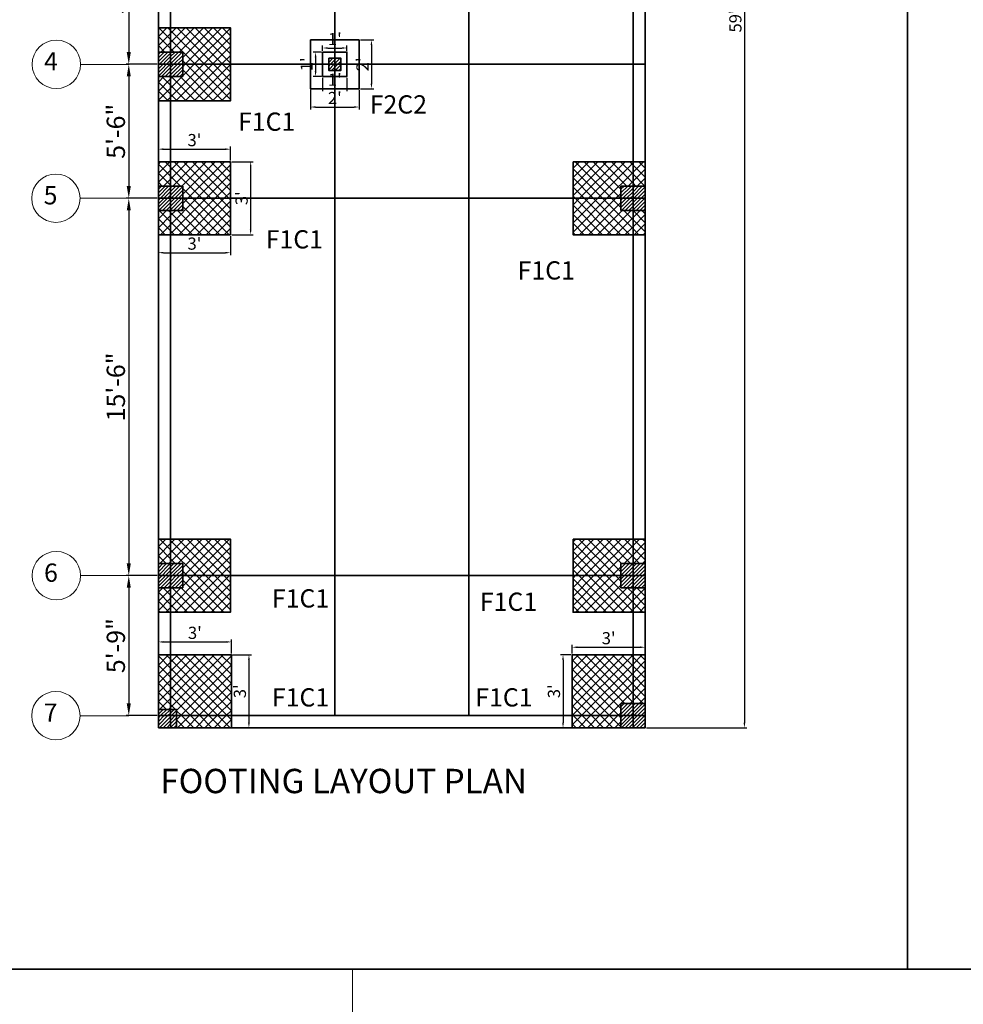
# Model space of a CAD drawing. Units: millimetres. Extents: x 20768 to 23556, y 50760 to 52704.
# Tile 33 of 36: x 22556 to 23021, y 51606 to 52092. Entities that reach past the tile are written whole.
import ezdxf

# ---------------------------------------------------------------- set-up
doc = ezdxf.new("R2010")
doc.units = ezdxf.units.MM
for name, color, linetype, lineweight in [('A-ANNO-SCHD', 7, 'Continuous', 18), ('A-ANNO-TTLB', 7, 'Continuous', 35), ('S-ANNO-DIMS', 2, 'Continuous', 18), ('S-ANNO-TEXT', 6, 'Continuous', 18), ('S-BEAM', 3, 'Continuous', 35), ('S-COLS', 20, 'Continuous', 35), ('S-COLS-PATT', 8, 'Continuous', 13), ('S-FNDN', 200, 'Continuous', 35), ('S-GRID', 1, 'Continuous', 18)]:
    doc.layers.add(name, color=color, linetype=linetype, lineweight=lineweight)
doc.styles.get("Standard").update_dxf_attribs({"font": 'arial.ttf'})
doc.dimstyles.new('ISO-25', dxfattribs={"dimtxt": 6, "dimasz": 2.5, "dimexe": 1.25, "dimexo": 0.625, "dimtad": 1, "dimdec": 0, "dimlunit": 3, "dimtxsty": 'Standard', "dimcen": 2.5, "dimadec": 0, "dimazin": 0, "dimtfac": 1, "dimtdec": 0, "dimtmove": 0, "dimatfit": 3, "dimfxl": 1, "dimarcsym": 0})
pattern_1 = [(45, (568.6884, 0), (-0.898025612, 0.898025612), [])]
pattern_2 = [(45, (-102.8262, 0), (-2.24506403, 2.24506403), []), (135, (-102.8262, 0), (-2.24506403, -2.24506403), [])]
pattern_3 = [(45, (-102.8262, 0), (-0.898025612, 0.898025612), [])]

# ---------------------------------------------------------------- blocks, each defined once
blk = doc.blocks.new('*D56')
at = {"layer": 'Defpoints', "color": 0, "transparency": 16777216}
for p in [(22623.96, 52129.51), (22609.39, 52069.51), (22623.96, 52069.51)]:
    blk.add_point(p, dxfattribs=at)
at = {"layer": 'S-ANNO-DIMS', "color": 0, "lineweight": -2, "transparency": 16777216}
for p, q in [((22623.34, 52129.51), (22608.14, 52129.51)), ((22609.39, 52123.51), (22609.39, 52075.51)), ((22623.34, 52069.51), (22608.14, 52069.51))]:
    blk.add_line(p, q, dxfattribs=at)
at = {"layer": 'S-ANNO-DIMS', "color": 0, "transparency": 16777216}
for points in [[(22608.39, 52123.51), (22610.39, 52123.51), (22609.39, 52129.51)], [(22608.39, 52075.51), (22610.39, 52075.51), (22609.39, 52069.51)]]:
    blk.add_solid(points, dxfattribs=at)
at = {"layer": 'S-ANNO-DIMS', "color": 0, "transparency": 16777216, "insert": (22604.19, 52099.51), "char_height": 9, "attachment_point": 5, "rotation": 90}
blk.add_mtext("5'", dxfattribs=at)
blk = doc.blocks.new('*D57')
at = {"layer": 'Defpoints', "color": 0, "transparency": 16777216}
for p in [(22623.96, 52069.51), (22609.39, 52003.51), (22623.96, 52003.51)]:
    blk.add_point(p, dxfattribs=at)
at = {"layer": 'S-ANNO-DIMS', "color": 0, "lineweight": -2, "transparency": 16777216}
for p, q in [((22623.34, 52069.51), (22608.14, 52069.51)), ((22609.39, 52063.51), (22609.39, 52009.51)), ((22623.34, 52003.51), (22608.14, 52003.51))]:
    blk.add_line(p, q, dxfattribs=at)
at = {"layer": 'S-ANNO-DIMS', "color": 0, "transparency": 16777216}
for points in [[(22608.39, 52063.51), (22610.39, 52063.51), (22609.39, 52069.51)], [(22608.39, 52009.51), (22610.39, 52009.51), (22609.39, 52003.51)]]:
    blk.add_solid(points, dxfattribs=at)
at = {"layer": 'S-ANNO-DIMS', "color": 0, "transparency": 16777216, "insert": (22604.17, 52036.51), "char_height": 9, "attachment_point": 5, "rotation": 90}
blk.add_mtext('5\'-6"', dxfattribs=at)
blk = doc.blocks.new('*D58')
at = {"layer": 'Defpoints', "color": 0, "transparency": 16777216}
for p in [(22623.96, 52003.51), (22609.39, 51817.51), (22623.96, 51817.51)]:
    blk.add_point(p, dxfattribs=at)
at = {"layer": 'S-ANNO-DIMS', "color": 0, "lineweight": -2, "transparency": 16777216}
for p, q in [((22623.34, 52003.51), (22608.14, 52003.51)), ((22609.39, 51997.51), (22609.39, 51823.51)), ((22623.34, 51817.51), (22608.14, 51817.51))]:
    blk.add_line(p, q, dxfattribs=at)
at = {"layer": 'S-ANNO-DIMS', "color": 0, "transparency": 16777216}
for points in [[(22608.39, 51997.51), (22610.39, 51997.51), (22609.39, 52003.51)], [(22608.39, 51823.51), (22610.39, 51823.51), (22609.39, 51817.51)]]:
    blk.add_solid(points, dxfattribs=at)
at = {"layer": 'S-ANNO-DIMS', "color": 0, "transparency": 16777216, "insert": (22604.17, 51910.51), "char_height": 9, "attachment_point": 5, "rotation": 90}
blk.add_mtext('15\'-6"', dxfattribs=at)
blk = doc.blocks.new('*D47')
at = {"layer": 'Defpoints', "color": 0, "transparency": 16777216}
for p in [(22623.96, 51817.51), (22609.39, 51748.51), (22623.96, 51748.51)]:
    blk.add_point(p, dxfattribs=at)
at = {"layer": 'S-ANNO-DIMS', "color": 0, "lineweight": -2, "transparency": 16777216}
for p, q in [((22623.34, 51817.51), (22608.14, 51817.51)), ((22609.39, 51811.51), (22609.39, 51754.51)), ((22623.34, 51748.51), (22608.14, 51748.51))]:
    blk.add_line(p, q, dxfattribs=at)
at = {"layer": 'S-ANNO-DIMS', "color": 0, "transparency": 16777216}
for points in [[(22608.39, 51811.51), (22610.39, 51811.51), (22609.39, 51817.51)], [(22608.39, 51754.51), (22610.39, 51754.51), (22609.39, 51748.51)]]:
    blk.add_solid(points, dxfattribs=at)
at = {"layer": 'S-ANNO-DIMS', "color": 0, "transparency": 16777216, "insert": (22604.17, 51783.01), "char_height": 9, "attachment_point": 5, "rotation": 90}
blk.add_mtext('5\'-9"', dxfattribs=at)
blk = doc.blocks.new('*D68')
at = {"layer": 'Defpoints', "color": 0, "transparency": 16777216}
for p in [(22704.96, 52075.51), (22716.96, 52077.55), (22716.96, 52075.51)]:
    blk.add_point(p, dxfattribs=at)
at = {"layer": 'S-ANNO-DIMS', "color": 0, "lineweight": -2, "transparency": 16777216}
for p, q in [((22704.96, 52076.13), (22704.96, 52078.8)), ((22716.96, 52076.13), (22716.96, 52078.8)), ((22707.46, 52077.55), (22714.46, 52077.55))]:
    blk.add_line(p, q, dxfattribs=at)
at = {"layer": 'S-ANNO-DIMS', "color": 0, "transparency": 16777216}
for points in [[(22707.46, 52077.96), (22707.46, 52077.13), (22704.96, 52077.55)], [(22714.46, 52077.96), (22714.46, 52077.13), (22716.96, 52077.55)]]:
    blk.add_solid(points, dxfattribs=at)
at = {"layer": 'S-ANNO-DIMS', "color": 0, "transparency": 16777216, "insert": (22710.96, 52081.18), "char_height": 6, "attachment_point": 5}
blk.add_mtext("1'", dxfattribs=at)
blk = doc.blocks.new('*D69')
at = {"layer": 'Defpoints', "color": 0, "transparency": 16777216}
for p in [(22722.96, 52081.51), (22722.96, 52057.51), (22729.01, 52057.51)]:
    blk.add_point(p, dxfattribs=at)
at = {"layer": 'S-ANNO-DIMS', "color": 0, "lineweight": -2, "transparency": 16777216}
for p, q in [((22723.59, 52081.51), (22730.26, 52081.51)), ((22729.01, 52079.01), (22729.01, 52060.01)), ((22723.59, 52057.51), (22730.26, 52057.51))]:
    blk.add_line(p, q, dxfattribs=at)
at = {"layer": 'S-ANNO-DIMS', "color": 0, "transparency": 16777216}
for points in [[(22728.59, 52079.01), (22729.42, 52079.01), (22729.01, 52081.51)], [(22728.59, 52060.01), (22729.42, 52060.01), (22729.01, 52057.51)]]:
    blk.add_solid(points, dxfattribs=at)
at = {"layer": 'S-ANNO-DIMS', "color": 0, "transparency": 16777216, "insert": (22725.37, 52069.51), "char_height": 6, "attachment_point": 5, "rotation": 90}
blk.add_mtext("2'", dxfattribs=at)
blk = doc.blocks.new('*D70')
at = {"layer": 'Defpoints', "color": 0, "transparency": 16777216}
for p in [(22698.96, 52057.51), (22722.96, 52057.51), (22722.96, 52048.47)]:
    blk.add_point(p, dxfattribs=at)
at = {"layer": 'S-ANNO-DIMS', "color": 0, "lineweight": -2, "transparency": 16777216}
for p, q in [((22698.96, 52056.88), (22698.96, 52047.22)), ((22722.96, 52056.88), (22722.96, 52047.22)), ((22701.46, 52048.47), (22720.46, 52048.47))]:
    blk.add_line(p, q, dxfattribs=at)
at = {"layer": 'S-ANNO-DIMS', "color": 0, "transparency": 16777216}
for points in [[(22701.46, 52048.89), (22701.46, 52048.06), (22698.96, 52048.47)], [(22720.46, 52048.89), (22720.46, 52048.06), (22722.96, 52048.47)]]:
    blk.add_solid(points, dxfattribs=at)
at = {"layer": 'S-ANNO-DIMS', "color": 0, "transparency": 16777216, "insert": (22710.96, 52052.11), "char_height": 6, "attachment_point": 5}
blk.add_mtext("2'", dxfattribs=at)
blk = doc.blocks.new('*D71')
at = {"layer": 'Defpoints', "color": 0, "transparency": 16777216}
for p in [(22704.96, 52063.51), (22716.96, 52063.51), (22716.96, 52057.51)]:
    blk.add_point(p, dxfattribs=at)
at = {"layer": 'S-ANNO-DIMS', "color": 0, "lineweight": -2, "transparency": 16777216}
for p, q in [((22704.96, 52062.88), (22704.96, 52056.26)), ((22716.96, 52062.88), (22716.96, 52056.26)), ((22707.46, 52057.51), (22714.46, 52057.51))]:
    blk.add_line(p, q, dxfattribs=at)
at = {"layer": 'S-ANNO-DIMS', "color": 0, "transparency": 16777216}
for points in [[(22707.46, 52057.93), (22707.46, 52057.09), (22704.96, 52057.51)], [(22714.46, 52057.93), (22714.46, 52057.09), (22716.96, 52057.51)]]:
    blk.add_solid(points, dxfattribs=at)
at = {"layer": 'S-ANNO-DIMS', "color": 0, "transparency": 16777216, "insert": (22710.96, 52061.15), "char_height": 6, "attachment_point": 5}
blk.add_mtext("1'", dxfattribs=at)
blk = doc.blocks.new('*D50')
at = {"layer": 'Defpoints', "color": 0, "transparency": 16777216}
for p in [(22704.96, 52075.51), (22701.48, 52063.51), (22704.96, 52063.51)]:
    blk.add_point(p, dxfattribs=at)
at = {"layer": 'S-ANNO-DIMS', "color": 0, "lineweight": -2, "transparency": 16777216}
for p, q in [((22704.34, 52075.51), (22700.23, 52075.51)), ((22701.48, 52073.01), (22701.48, 52066.01)), ((22704.34, 52063.51), (22700.23, 52063.51))]:
    blk.add_line(p, q, dxfattribs=at)
at = {"layer": 'S-ANNO-DIMS', "color": 0, "transparency": 16777216}
for points in [[(22701.07, 52073.01), (22701.9, 52073.01), (22701.48, 52075.51)], [(22701.07, 52066.01), (22701.9, 52066.01), (22701.48, 52063.51)]]:
    blk.add_solid(points, dxfattribs=at)
at = {"layer": 'S-ANNO-DIMS', "color": 0, "transparency": 16777216, "insert": (22697.85, 52069.51), "char_height": 6, "attachment_point": 5, "rotation": 90}
blk.add_mtext("1'", dxfattribs=at)
blk = doc.blocks.new('*D72')
at = {"layer": 'Defpoints', "color": 0, "transparency": 16777216}
for p in [(22659.96, 51784.85), (22623.96, 51778.51), (22659.96, 51778.51)]:
    blk.add_point(p, dxfattribs=at)
at = {"layer": 'S-ANNO-DIMS', "color": 0, "lineweight": -2, "transparency": 16777216}
for p, q in [((22623.96, 51779.13), (22623.96, 51786.1)), ((22626.46, 51784.85), (22657.46, 51784.85)), ((22659.96, 51779.13), (22659.96, 51786.1))]:
    blk.add_line(p, q, dxfattribs=at)
at = {"layer": 'S-ANNO-DIMS', "color": 0, "transparency": 16777216}
for points in [[(22626.46, 51785.26), (22626.46, 51784.43), (22623.96, 51784.85)], [(22657.46, 51785.26), (22657.46, 51784.43), (22659.96, 51784.85)]]:
    blk.add_solid(points, dxfattribs=at)
at = {"layer": 'S-ANNO-DIMS', "color": 0, "transparency": 16777216, "insert": (22641.96, 51788.54), "char_height": 6, "attachment_point": 5}
blk.add_mtext("3'", dxfattribs=at)
blk = doc.blocks.new('*D73')
at = {"layer": 'Defpoints', "color": 0, "transparency": 16777216}
for p in [(22659.96, 51778.51), (22659.96, 51742.51), (22668.62, 51742.51)]:
    blk.add_point(p, dxfattribs=at)
at = {"layer": 'S-ANNO-DIMS', "color": 0, "lineweight": -2, "transparency": 16777216}
for p, q in [((22660.59, 51778.51), (22669.87, 51778.51)), ((22668.62, 51776.01), (22668.62, 51745.01)), ((22660.59, 51742.51), (22669.87, 51742.51))]:
    blk.add_line(p, q, dxfattribs=at)
at = {"layer": 'S-ANNO-DIMS', "color": 0, "transparency": 16777216}
for points in [[(22668.2, 51776.01), (22669.04, 51776.01), (22668.62, 51778.51)], [(22668.2, 51745.01), (22669.04, 51745.01), (22668.62, 51742.51)]]:
    blk.add_solid(points, dxfattribs=at)
at = {"layer": 'S-ANNO-DIMS', "color": 0, "transparency": 16777216, "insert": (22664.93, 51760.51), "char_height": 6, "attachment_point": 5, "rotation": 90}
blk.add_mtext("3'", dxfattribs=at)
blk = doc.blocks.new('*D74')
at = {"layer": 'Defpoints', "color": 0, "transparency": 16777216}
for p in [(22863.96, 51782.23), (22827.96, 51778.51), (22863.96, 51778.51)]:
    blk.add_point(p, dxfattribs=at)
at = {"layer": 'S-ANNO-DIMS', "color": 0, "lineweight": -2, "transparency": 16777216}
for p, q in [((22827.96, 51779.13), (22827.96, 51783.48)), ((22830.46, 51782.23), (22861.46, 51782.23)), ((22863.96, 51779.13), (22863.96, 51783.48))]:
    blk.add_line(p, q, dxfattribs=at)
at = {"layer": 'S-ANNO-DIMS', "color": 0, "transparency": 16777216}
for points in [[(22830.46, 51782.64), (22830.46, 51781.81), (22827.96, 51782.23)], [(22861.46, 51782.64), (22861.46, 51781.81), (22863.96, 51782.23)]]:
    blk.add_solid(points, dxfattribs=at)
at = {"layer": 'S-ANNO-DIMS', "color": 0, "transparency": 16777216, "insert": (22845.96, 51785.92), "char_height": 6, "attachment_point": 5}
blk.add_mtext("3'", dxfattribs=at)
blk = doc.blocks.new('*D75')
at = {"layer": 'Defpoints', "color": 0, "transparency": 16777216}
for p in [(22827.96, 51778.51), (22823.46, 51742.51), (22827.96, 51742.51)]:
    blk.add_point(p, dxfattribs=at)
at = {"layer": 'S-ANNO-DIMS', "color": 0, "lineweight": -2, "transparency": 16777216}
for p, q in [((22827.34, 51778.51), (22822.21, 51778.51)), ((22823.46, 51776.01), (22823.46, 51745.01)), ((22827.34, 51742.51), (22822.21, 51742.51))]:
    blk.add_line(p, q, dxfattribs=at)
at = {"layer": 'S-ANNO-DIMS', "color": 0, "transparency": 16777216}
for points in [[(22823.04, 51776.01), (22823.88, 51776.01), (22823.46, 51778.51)], [(22823.04, 51745.01), (22823.88, 51745.01), (22823.46, 51742.51)]]:
    blk.add_solid(points, dxfattribs=at)
at = {"layer": 'S-ANNO-DIMS', "color": 0, "transparency": 16777216, "insert": (22819.77, 51760.51), "char_height": 6, "attachment_point": 5, "rotation": 90}
blk.add_mtext("3'", dxfattribs=at)
blk = doc.blocks.new('*D76')
at = {"layer": 'Defpoints', "color": 0, "transparency": 16777216}
for p in [(22659.53, 52027.69), (22623.96, 52021.51), (22659.53, 52021.51)]:
    blk.add_point(p, dxfattribs=at)
at = {"layer": 'S-ANNO-DIMS', "color": 0, "lineweight": -2, "transparency": 16777216}
for p, q in [((22623.96, 52022.13), (22623.96, 52028.94)), ((22626.46, 52027.69), (22657.03, 52027.69)), ((22659.53, 52022.13), (22659.53, 52028.94))]:
    blk.add_line(p, q, dxfattribs=at)
at = {"layer": 'S-ANNO-DIMS', "color": 0, "transparency": 16777216}
for points in [[(22626.46, 52028.11), (22626.46, 52027.28), (22623.96, 52027.69)], [(22657.03, 52028.11), (22657.03, 52027.28), (22659.53, 52027.69)]]:
    blk.add_solid(points, dxfattribs=at)
at = {"layer": 'S-ANNO-DIMS', "color": 0, "transparency": 16777216, "insert": (22641.75, 52031.39), "char_height": 6, "attachment_point": 5}
blk.add_mtext("3'", dxfattribs=at)
blk = doc.blocks.new('*D77')
at = {"layer": 'Defpoints', "color": 0, "transparency": 16777216}
for p in [(22659.53, 52021.51), (22659.53, 51985.51), (22669.47, 51985.51)]:
    blk.add_point(p, dxfattribs=at)
at = {"layer": 'S-ANNO-DIMS', "color": 0, "lineweight": -2, "transparency": 16777216}
for p, q in [((22660.16, 52021.51), (22670.72, 52021.51)), ((22669.47, 52019.01), (22669.47, 51988.01)), ((22660.16, 51985.51), (22670.72, 51985.51))]:
    blk.add_line(p, q, dxfattribs=at)
at = {"layer": 'S-ANNO-DIMS', "color": 0, "transparency": 16777216}
for points in [[(22669.05, 52019.01), (22669.89, 52019.01), (22669.47, 52021.51)], [(22669.05, 51988.01), (22669.89, 51988.01), (22669.47, 51985.51)]]:
    blk.add_solid(points, dxfattribs=at)
at = {"layer": 'S-ANNO-DIMS', "color": 0, "transparency": 16777216, "insert": (22665.78, 52003.51), "char_height": 6, "attachment_point": 5, "rotation": 90}
blk.add_mtext("3'", dxfattribs=at)
blk = doc.blocks.new('*D78')
at = {"layer": 'Defpoints', "color": 0, "transparency": 16777216}
for p in [(22623.96, 51985.51), (22659.53, 51985.51), (22659.53, 51976.68)]:
    blk.add_point(p, dxfattribs=at)
at = {"layer": 'S-ANNO-DIMS', "color": 0, "lineweight": -2, "transparency": 16777216}
for p, q in [((22623.96, 51984.88), (22623.96, 51975.43)), ((22659.53, 51984.88), (22659.53, 51975.43)), ((22626.46, 51976.68), (22657.03, 51976.68))]:
    blk.add_line(p, q, dxfattribs=at)
at = {"layer": 'S-ANNO-DIMS', "color": 0, "transparency": 16777216}
for points in [[(22626.46, 51977.1), (22626.46, 51976.27), (22623.96, 51976.68)], [(22657.03, 51977.1), (22657.03, 51976.27), (22659.53, 51976.68)]]:
    blk.add_solid(points, dxfattribs=at)
at = {"layer": 'S-ANNO-DIMS', "color": 0, "transparency": 16777216, "insert": (22641.75, 51980.37), "char_height": 6, "attachment_point": 5}
blk.add_mtext("3'", dxfattribs=at)
blk = doc.blocks.new('GRID-BUBBLE')
blk.add_line((47.87, 11.93), (23.87, 11.93))
blk.add_circle((11.93, 11.93), 11.93)
blk = doc.blocks.new('*D226')
at = {"layer": 'Defpoints', "color": 0, "transparency": 16777216}
for p in [(22863.96, 52450.51), (22863.96, 51742.51), (22912.89, 51742.51)]:
    blk.add_point(p, dxfattribs=at)
at = {"layer": 'S-ANNO-DIMS', "color": 0, "lineweight": -2, "transparency": 16777216}
for p, q in [((22864.59, 52450.51), (22914.14, 52450.51)), ((22912.89, 52448.01), (22912.89, 51745.01)), ((22864.59, 51742.51), (22914.14, 51742.51))]:
    blk.add_line(p, q, dxfattribs=at)
at = {"layer": 'S-ANNO-DIMS', "color": 0, "transparency": 16777216}
for points in [[(22912.48, 52448.01), (22913.31, 52448.01), (22912.89, 52450.51)], [(22912.48, 51745.01), (22913.31, 51745.01), (22912.89, 51742.51)]]:
    blk.add_solid(points, dxfattribs=at)
at = {"layer": 'S-ANNO-DIMS', "color": 0, "transparency": 16777216, "insert": (22909.21, 52096.51), "char_height": 6, "attachment_point": 5, "rotation": 90}
blk.add_mtext('59\'-0"', dxfattribs=at)

msp = doc.modelspace()

# ---------------------------------------------------------------- hatches: boundary and pattern name
at = {"layer": 'S-COLS-PATT'}
h = msp.add_hatch(dxfattribs=at)
h.set_pattern_fill('ANSI37', color=256)
h.set_pattern_definition(pattern_2)
h.paths.add_polyline_path([(22629.96, 52087.51), (22623.96, 52087.51), (22623.96, 52075.51), (22629.96, 52075.51)])
h = msp.add_hatch(dxfattribs=at)
h.set_pattern_fill('ANSI37', color=256)
h.set_pattern_definition(pattern_2)
h.paths.add_polyline_path([(22659.53, 52087.51), (22629.96, 52087.51), (22629.96, 52075.51), (22635.96, 52075.51), (22635.96, 52069.51), (22659.53, 52069.51)])
h = msp.add_hatch(dxfattribs=at)
h.set_pattern_fill('ANSI31', color=256, scale=0.4)
h.set_pattern_definition(pattern_1)
h.paths.add_polyline_path([(22629.96, 52075.51), (22623.96, 52075.51), (22623.96, 52063.51), (22629.96, 52063.51)])
h = msp.add_hatch(dxfattribs=at)
h.set_pattern_fill('ANSI31', color=256, scale=0.4)
h.set_pattern_definition(pattern_1)
h.paths.add_polyline_path([(22635.96, 52075.51), (22629.96, 52075.51), (22629.96, 52069.51), (22635.96, 52069.51)])
h = msp.add_hatch(dxfattribs=at)
h.set_pattern_fill('ANSI31', color=256, scale=0.4)
h.set_pattern_definition(pattern_1)
h.paths.add_polyline_path([(22635.96, 52069.51), (22629.96, 52069.51), (22629.96, 52063.51), (22635.96, 52063.51)])
h = msp.add_hatch(dxfattribs=at)
h.set_pattern_fill('ANSI37', color=256)
h.set_pattern_definition(pattern_2)
h.paths.add_polyline_path([(22659.53, 52069.51), (22635.96, 52069.51), (22635.96, 52063.51), (22629.96, 52063.51), (22629.96, 52051.51), (22659.53, 52051.51)])
h = msp.add_hatch(dxfattribs=at)
h.set_pattern_fill('ANSI31', color=256, scale=0.4)
h.set_pattern_definition(pattern_1)
h.paths.add_polyline_path([(22710.96, 52072.51), (22707.96, 52072.51), (22707.96, 52069.51), (22710.96, 52069.51)])
h = msp.add_hatch(dxfattribs=at)
h.set_pattern_fill('ANSI31', color=256, scale=0.4)
h.set_pattern_definition(pattern_1)
h.paths.add_polyline_path([(22710.96, 52069.51), (22707.96, 52069.51), (22707.96, 52066.51), (22710.96, 52066.51)])
h = msp.add_hatch(dxfattribs=at)
h.set_pattern_fill('ANSI31', color=256, scale=0.4)
h.set_pattern_definition(pattern_1)
h.paths.add_polyline_path([(22713.96, 52072.51), (22710.96, 52072.51), (22710.96, 52069.51), (22713.96, 52069.51)], flags=17)
h = msp.add_hatch(dxfattribs=at)
h.set_pattern_fill('ANSI31', color=256, scale=0.4)
h.set_pattern_definition(pattern_1)
h.paths.add_polyline_path([(22713.96, 52069.51), (22710.96, 52069.51), (22710.96, 52066.51), (22713.96, 52066.51)])
h = msp.add_hatch(dxfattribs=at)
h.set_pattern_fill('ANSI37', color=256)
h.set_pattern_definition(pattern_2)
h.paths.add_polyline_path([(22629.96, 52063.51), (22623.96, 52063.51), (22623.96, 52051.51), (22629.96, 52051.51)])
h = msp.add_hatch(dxfattribs=at)
h.set_pattern_fill('ANSI37', color=256)
h.set_pattern_definition(pattern_2)
h.paths.add_polyline_path([(22629.96, 52021.51), (22623.96, 52021.51), (22623.96, 52009.51), (22629.96, 52009.51)])
h = msp.add_hatch(dxfattribs=at)
h.set_pattern_fill('ANSI37', color=256)
h.set_pattern_definition(pattern_2)
h.paths.add_polyline_path([(22659.53, 52021.51), (22629.96, 52021.51), (22629.96, 52009.51), (22635.96, 52009.51), (22635.96, 52003.51), (22659.53, 52003.51)])
h = msp.add_hatch(dxfattribs=at)
h.set_pattern_fill('ANSI37', color=256)
h.set_pattern_definition(pattern_2)
h.paths.add_polyline_path([(22857.96, 52021.51), (22828.39, 52021.51), (22828.39, 52003.51), (22851.96, 52003.51), (22851.96, 52009.51), (22857.96, 52009.51)])
h = msp.add_hatch(dxfattribs=at)
h.set_pattern_fill('ANSI37', color=256)
h.set_pattern_definition(pattern_2)
h.paths.add_polyline_path([(22863.96, 52021.51), (22857.96, 52021.51), (22857.96, 52009.51), (22863.96, 52009.51)])
h = msp.add_hatch(dxfattribs=at)
h.set_pattern_fill('ANSI31', color=256, scale=0.4)
h.set_pattern_definition(pattern_1)
h.paths.add_polyline_path([(22629.96, 52009.51), (22623.96, 52009.51), (22623.96, 51997.51), (22629.96, 51997.51)])
h = msp.add_hatch(dxfattribs=at)
h.set_pattern_fill('ANSI31', color=256, scale=0.4)
h.set_pattern_definition(pattern_1)
h.paths.add_polyline_path([(22635.96, 52009.51), (22629.96, 52009.51), (22629.96, 52003.51), (22635.96, 52003.51)])
h = msp.add_hatch(dxfattribs=at)
h.set_pattern_fill('ANSI31', color=256, scale=0.4)
h.set_pattern_definition(pattern_1)
h.paths.add_polyline_path([(22857.96, 52009.51), (22851.96, 52009.51), (22851.96, 52003.51), (22857.96, 52003.51)])
h = msp.add_hatch(dxfattribs=at)
h.set_pattern_fill('ANSI31', color=256, scale=0.4)
h.set_pattern_definition(pattern_1)
h.paths.add_polyline_path([(22863.96, 52009.51), (22857.96, 52009.51), (22857.96, 52003.51), (22863.96, 52003.51)])
h = msp.add_hatch(dxfattribs=at)
h.set_pattern_fill('ANSI31', color=256, scale=0.4)
h.set_pattern_definition(pattern_1)
h.paths.add_polyline_path([(22635.96, 52003.51), (22629.96, 52003.51), (22629.96, 51997.51), (22635.96, 51997.51)])
h = msp.add_hatch(dxfattribs=at)
h.set_pattern_fill('ANSI37', color=256)
h.set_pattern_definition(pattern_2)
h.paths.add_polyline_path([(22659.53, 52003.51), (22635.96, 52003.51), (22635.96, 51997.51), (22629.96, 51997.51), (22629.96, 51985.51), (22659.53, 51985.51)])
h = msp.add_hatch(dxfattribs=at)
h.set_pattern_fill('ANSI37', color=256)
h.set_pattern_definition(pattern_2)
h.paths.add_polyline_path([(22857.96, 51997.51), (22851.96, 51997.51), (22851.96, 52003.51), (22828.39, 52003.51), (22828.39, 51985.51), (22857.96, 51985.51)])
h = msp.add_hatch(dxfattribs=at)
h.set_pattern_fill('ANSI31', color=256, scale=0.4)
h.set_pattern_definition(pattern_1)
h.paths.add_polyline_path([(22857.96, 52003.51), (22851.96, 52003.51), (22851.96, 51997.51), (22857.96, 51997.51)])
h = msp.add_hatch(dxfattribs=at)
h.set_pattern_fill('ANSI31', color=256, scale=0.4)
h.set_pattern_definition(pattern_1)
h.paths.add_polyline_path([(22863.96, 52003.51), (22857.96, 52003.51), (22857.96, 51997.51), (22863.96, 51997.51)])
h = msp.add_hatch(dxfattribs=at)
h.set_pattern_fill('ANSI37', color=256)
h.set_pattern_definition(pattern_2)
h.paths.add_polyline_path([(22629.96, 51997.51), (22623.96, 51997.51), (22623.96, 51985.51), (22629.96, 51985.51)])
h = msp.add_hatch(dxfattribs=at)
h.set_pattern_fill('ANSI37', color=256)
h.set_pattern_definition(pattern_2)
h.paths.add_polyline_path([(22863.96, 51997.51), (22857.96, 51997.51), (22857.96, 51985.51), (22863.96, 51985.51)])
h = msp.add_hatch(dxfattribs=at)
h.set_pattern_fill('ANSI37', color=256)
h.set_pattern_definition(pattern_2)
h.paths.add_polyline_path([(22629.96, 51835.51), (22623.96, 51835.51), (22623.96, 51823.51), (22629.96, 51823.51)])
h = msp.add_hatch(dxfattribs=at)
h.set_pattern_fill('ANSI37', color=256)
h.set_pattern_definition(pattern_2)
h.paths.add_polyline_path([(22659.53, 51835.51), (22629.96, 51835.51), (22629.96, 51823.51), (22635.96, 51823.51), (22635.96, 51817.51), (22659.53, 51817.51)])
h = msp.add_hatch(dxfattribs=at)
h.set_pattern_fill('ANSI37', color=256)
h.set_pattern_definition(pattern_2)
h.paths.add_polyline_path([(22857.96, 51835.51), (22828.39, 51835.51), (22828.39, 51817.51), (22851.96, 51817.51), (22851.96, 51823.51), (22857.96, 51823.51)])
h = msp.add_hatch(dxfattribs=at)
h.set_pattern_fill('ANSI37', color=256)
h.set_pattern_definition(pattern_2)
h.paths.add_polyline_path([(22863.96, 51835.51), (22857.96, 51835.51), (22857.96, 51823.51), (22863.96, 51823.51)])
h = msp.add_hatch(dxfattribs=at)
h.set_pattern_fill('ANSI31', color=256, scale=0.4)
h.set_pattern_definition(pattern_1)
h.paths.add_polyline_path([(22629.96, 51823.51), (22623.96, 51823.51), (22623.96, 51811.51), (22629.96, 51811.51)])
h = msp.add_hatch(dxfattribs=at)
h.set_pattern_fill('ANSI31', color=256, scale=0.4)
h.set_pattern_definition(pattern_1)
h.paths.add_polyline_path([(22635.96, 51823.51), (22629.96, 51823.51), (22629.96, 51817.51), (22635.96, 51817.51)])
h = msp.add_hatch(dxfattribs=at)
h.set_pattern_fill('ANSI31', color=256, scale=0.4)
h.set_pattern_definition(pattern_1)
h.paths.add_polyline_path([(22863.96, 51823.51), (22851.96, 51823.51), (22851.96, 51811.51), (22863.96, 51811.51)])
h = msp.add_hatch(dxfattribs=at)
h.set_pattern_fill('ANSI31', color=256, scale=0.4)
h.set_pattern_definition(pattern_1)
h.paths.add_polyline_path([(22635.96, 51817.51), (22629.96, 51817.51), (22629.96, 51811.51), (22635.96, 51811.51)])
h = msp.add_hatch(dxfattribs=at)
h.set_pattern_fill('ANSI37', color=256)
h.set_pattern_definition(pattern_2)
h.paths.add_polyline_path([(22659.53, 51817.51), (22635.96, 51817.51), (22635.96, 51811.51), (22629.96, 51811.51), (22629.96, 51799.51), (22659.53, 51799.51)])
h = msp.add_hatch(dxfattribs=at)
h.set_pattern_fill('ANSI37', color=256)
h.set_pattern_definition(pattern_2)
h.paths.add_polyline_path([(22857.96, 51811.51), (22851.96, 51811.51), (22851.96, 51817.51), (22828.39, 51817.51), (22828.39, 51799.51), (22857.96, 51799.51)])
h = msp.add_hatch(dxfattribs=at)
h.set_pattern_fill('ANSI37', color=256)
h.set_pattern_definition(pattern_2)
h.paths.add_polyline_path([(22629.96, 51811.51), (22623.96, 51811.51), (22623.96, 51799.51), (22629.96, 51799.51)])
h = msp.add_hatch(dxfattribs=at)
h.set_pattern_fill('ANSI37', color=256)
h.set_pattern_definition(pattern_2)
h.paths.add_polyline_path([(22863.96, 51811.51), (22857.96, 51811.51), (22857.96, 51799.51), (22863.96, 51799.51)])
h = msp.add_hatch(dxfattribs=at)
h.set_pattern_fill('ANSI37', color=256)
h.set_pattern_definition(pattern_2)
h.paths.add_polyline_path([(22629.96, 51778.51), (22623.96, 51778.51), (22623.96, 51751.51), (22629.96, 51751.51)])
h = msp.add_hatch(dxfattribs=at)
h.set_pattern_fill('ANSI37', color=256)
h.set_pattern_definition(pattern_2)
h.paths.add_polyline_path([(22659.96, 51778.51), (22629.96, 51778.51), (22629.96, 51751.51), (22632.96, 51751.51), (22632.96, 51748.51), (22659.96, 51748.51)])
h = msp.add_hatch(dxfattribs=at)
h.set_pattern_fill('ANSI37', color=256)
h.set_pattern_definition(pattern_2)
h.paths.add_polyline_path([(22857.96, 51778.51), (22827.96, 51778.51), (22827.96, 51748.51), (22851.96, 51748.51), (22851.96, 51754.51), (22857.96, 51754.51)])
h = msp.add_hatch(dxfattribs=at)
h.set_pattern_fill('ANSI37', color=256)
h.set_pattern_definition(pattern_2)
h.paths.add_polyline_path([(22863.96, 51778.51), (22857.96, 51778.51), (22857.96, 51754.51), (22863.96, 51754.51)])
h = msp.add_hatch(dxfattribs=at)
h.set_pattern_fill('ANSI31', color=256, scale=0.4)
h.set_pattern_definition(pattern_1)
h.paths.add_polyline_path([(22863.96, 51754.51), (22851.96, 51754.51), (22851.96, 51742.51), (22863.96, 51742.51)])
h = msp.add_hatch(dxfattribs=at)
h.set_pattern_fill('ANSI31', color=256, scale=0.4)
h.set_pattern_definition(pattern_3)
h.paths.add_polyline_path([(22629.96, 51751.51), (22623.96, 51751.51), (22623.96, 51748.51), (22629.96, 51748.51)])
h = msp.add_hatch(dxfattribs=at)
h.set_pattern_fill('ANSI31', color=256, scale=0.4)
h.set_pattern_definition(pattern_3)
h.paths.add_polyline_path([(22629.96, 51748.51), (22623.96, 51748.51), (22623.96, 51742.51), (22629.96, 51742.51)])
h = msp.add_hatch(dxfattribs=at)
h.set_pattern_fill('ANSI31', color=256, scale=0.4)
h.set_pattern_definition(pattern_3)
h.paths.add_polyline_path([(22632.96, 51751.51), (22629.96, 51751.51), (22629.96, 51748.51), (22632.96, 51748.51)])
h = msp.add_hatch(dxfattribs=at)
h.set_pattern_fill('ANSI31', color=256, scale=0.4)
h.set_pattern_definition(pattern_3)
h.paths.add_polyline_path([(22632.96, 51748.51), (22629.96, 51748.51), (22629.96, 51742.51), (22632.96, 51742.51)])
h = msp.add_hatch(dxfattribs=at)
h.set_pattern_fill('ANSI37', color=256)
h.set_pattern_definition(pattern_2)
h.paths.add_polyline_path([(22659.96, 51748.51), (22632.96, 51748.51), (22632.96, 51742.51), (22659.96, 51742.51)])
h = msp.add_hatch(dxfattribs=at)
h.set_pattern_fill('ANSI37', color=256)
h.set_pattern_definition(pattern_2)
h.paths.add_polyline_path([(22851.96, 51748.51), (22827.96, 51748.51), (22827.96, 51742.51), (22851.96, 51742.51)])

# ---------------------------------------------------------------- linework, layer by layer
at = {"layer": 'A-ANNO-SCHD'}
msp.add_line((22719.7, 51623.53), (22719.7, 50975.78), dxfattribs=at)
at = {"layer": 'A-ANNO-TTLB'}
msp.add_line((22993.36, 52703.98), (22993.36, 51623.53), dxfattribs=at)
msp.add_lwpolyline([(20768.14, 52703.98), (23555.8, 52703.98), (23555.8, 51623.53), (20768.14, 51623.53)], close=True, dxfattribs=at)
at = {"layer": 'S-BEAM'}
for p, q in [((22710.96, 52450.51), (22710.96, 51748.51)), ((22776.96, 52450.51), (22776.96, 51748.51)), ((22629.96, 52444.51), (22629.96, 51742.51)), ((22857.96, 52135.51), (22857.96, 51823.51)), ((22623.96, 52069.51), (22863.96, 52069.51)), ((22623.96, 52003.51), (22863.96, 52003.51)), ((22857.96, 51823.51), (22857.96, 51742.51)), ((22623.96, 51817.51), (22863.96, 51817.51)), ((22623.96, 51748.51), (22863.96, 51748.51))]:
    msp.add_line(p, q, dxfattribs=at)
at = {"layer": 'S-COLS'}
for points in [[(22623.96, 52087.51), (22659.53, 52087.51), (22659.53, 52051.51), (22623.96, 52051.51)], [(22698.96, 52081.51), (22722.96, 52081.51), (22722.96, 52057.51), (22698.96, 52057.51)], [(22635.96, 52075.51), (22623.96, 52075.51), (22623.96, 52063.51), (22635.96, 52063.51)], [(22704.96, 52075.51), (22716.96, 52075.51), (22716.96, 52063.51), (22704.96, 52063.51)], [(22707.96, 52072.51), (22713.96, 52072.51), (22713.96, 52066.51), (22707.96, 52066.51)], [(22623.96, 52021.51), (22659.53, 52021.51), (22659.53, 51985.51), (22623.96, 51985.51)], [(22828.39, 52021.51), (22863.96, 52021.51), (22863.96, 51985.51), (22828.39, 51985.51)], [(22635.96, 52009.51), (22623.96, 52009.51), (22623.96, 51997.51), (22635.96, 51997.51)], [(22851.96, 52009.51), (22863.96, 52009.51), (22863.96, 51997.51), (22851.96, 51997.51)], [(22623.96, 51835.51), (22659.53, 51835.51), (22659.53, 51799.51), (22623.96, 51799.51)], [(22828.39, 51835.51), (22863.96, 51835.51), (22863.96, 51799.51), (22828.39, 51799.51)], [(22635.96, 51823.51), (22623.96, 51823.51), (22623.96, 51811.51), (22635.96, 51811.51)], [(22851.96, 51823.51), (22863.96, 51823.51), (22863.96, 51811.51), (22851.96, 51811.51)], [(22623.96, 51742.51), (22659.96, 51742.51), (22659.96, 51778.51), (22623.96, 51778.51)], [(22863.96, 51742.51), (22827.96, 51742.51), (22827.96, 51778.51), (22863.96, 51778.51)], [(22851.96, 51754.51), (22863.96, 51754.51), (22863.96, 51742.51), (22851.96, 51742.51)], [(22623.96, 51742.51), (22632.96, 51742.51), (22632.96, 51751.51), (22623.96, 51751.51)]]:
    msp.add_lwpolyline(points, close=True, dxfattribs=at)
at = {"layer": 'S-FNDN'}
for p, q in [((22623.96, 52450.51), (22623.96, 51742.51)), ((22863.96, 52450.51), (22863.96, 51742.51)), ((22623.96, 51742.51), (22863.96, 51742.51))]:
    msp.add_line(p, q, dxfattribs=at)

# ---------------------------------------------------------------- block references
at = {"layer": 'S-GRID'}
for p in [(22561.73, 52057.57), (22561.52, 51991.57), (22561.73, 51805.57), (22561.52, 51736.57)]:
    msp.add_blockref('GRID-BUBBLE', p, dxfattribs=at)

# ---------------------------------------------------------------- texts
at = {"layer": 'S-ANNO-TEXT', "attachment_point": 1}
for s, width, insert, char_height in [('  4', 27.5349, (22562.12, 52075.48), 9), ('F2C2', 26.4582, (22728.17, 52054.25), 9), ('F1C1', 26.4582, (22663.26, 52045.76), 9), ('  5', 27.5349, (22561.91, 52009.48), 9), ('F1C1', 26.4582, (22676.89, 51987.76), 9), ('F1C1', 26.4582, (22801.08, 51972.45), 9), ('  6', 27.5349, (22562.12, 51823.48), 9), ('F1C1', 26.4582, (22679.94, 51810.8), 9), ('F1C1', 26.4582, (22782.47, 51809.16), 9), ('F1C1', 26.4582, (22679.94, 51762.02), 9), ('F1C1', 26.4582, (22780.21, 51762.02), 9), ('  7', 27.5349, (22561.91, 51754.48), 9), ('FOOTING LAYOUT PLAN', 241.5904, (22624.93, 51722.3), 12)]:
    msp.add_mtext_dynamic_manual_height_columns(s, width=width, gutter_width=12.5, heights=[0], dxfattribs=dict(at, insert=insert, char_height=char_height))

# ---------------------------------------------------------------- dimensions: what is measured, and where the dimension line sits
at = {"layer": 'S-ANNO-DIMS'}
for base, p1, p2, override, picture, middle in [((22912.89, 51742.51), (22863.96, 52450.51), (22863.96, 51742.51), {"dimdec": 1, "dimlfac": 1, "dimrnd": 0, "dimzin": 1, "dimdsep": 46, "dimlunit": 4, "dimfrac": 2}, '*D226', (22909.21, 52096.51)), ((22609.39, 52069.51), (22623.96, 52129.51), (22623.96, 52069.51), {"dimtxt": 9, "dimasz": 6, "dimclrd": 0, "dimclre": 0, "dimclrt": 0}, '*D56', (22604.19, 52099.51)), ((22729.01, 52057.51), (22722.96, 52081.51), (22722.96, 52057.51), {"dimclrd": 0, "dimclre": 0, "dimclrt": 0}, '*D69', (22725.37, 52069.51)), ((22701.48, 52063.51), (22704.96, 52075.51), (22704.96, 52063.51), {"dimclrd": 0, "dimclre": 0, "dimclrt": 0}, '*D50', (22697.85, 52069.51)), ((22609.39, 52003.51), (22623.96, 52069.51), (22623.96, 52003.51), {"dimtxt": 9, "dimasz": 6, "dimclrd": 0, "dimclre": 0, "dimclrt": 0}, '*D57', (22604.17, 52036.51)), ((22669.47, 51985.51), (22659.53, 52021.51), (22659.53, 51985.51), {"dimclrd": 0, "dimclre": 0, "dimclrt": 0}, '*D77', (22665.78, 52003.51)), ((22609.39, 51817.51), (22623.96, 52003.51), (22623.96, 51817.51), {"dimtxt": 9, "dimasz": 6, "dimclrd": 0, "dimclre": 0, "dimclrt": 0}, '*D58', (22604.17, 51910.51)), ((22609.39, 51748.51), (22623.96, 51817.51), (22623.96, 51748.51), {"dimtxt": 9, "dimasz": 6, "dimclrd": 0, "dimclre": 0, "dimclrt": 0}, '*D47', (22604.17, 51783.01)), ((22668.62, 51742.51), (22659.96, 51778.51), (22659.96, 51742.51), {"dimclrd": 0, "dimclre": 0, "dimclrt": 0}, '*D73', (22664.93, 51760.51)), ((22823.46, 51742.51), (22827.96, 51778.51), (22827.96, 51742.51), {"dimclrd": 0, "dimclre": 0, "dimclrt": 0}, '*D75', (22819.77, 51760.51))]:
    dim = msp.add_linear_dim(base=base, p1=p1, p2=p2, angle=90, dimstyle='ISO-25', override=override, dxfattribs=at)
    dim.commit()
    dim.dimension.update_dxf_attribs({"geometry": picture, "text_midpoint": middle})
for base, p1, p2, picture, middle in [((22716.96, 52077.55), (22704.96, 52075.51), (22716.96, 52075.51), '*D68', (22710.96, 52081.18)), ((22716.96, 52057.51), (22704.96, 52063.51), (22716.96, 52063.51), '*D71', (22710.96, 52061.15)), ((22722.96, 52048.47), (22698.96, 52057.51), (22722.96, 52057.51), '*D70', (22710.96, 52052.11)), ((22659.53, 52027.69), (22623.96, 52021.51), (22659.53, 52021.51), '*D76', (22641.75, 52031.39)), ((22659.53, 51976.68), (22623.96, 51985.51), (22659.53, 51985.51), '*D78', (22641.75, 51980.37)), ((22659.96, 51784.85), (22623.96, 51778.51), (22659.96, 51778.51), '*D72', (22641.96, 51788.54)), ((22863.96, 51782.23), (22827.96, 51778.51), (22863.96, 51778.51), '*D74', (22845.96, 51785.92))]:
    dim = msp.add_linear_dim(base=base, p1=p1, p2=p2, dimstyle='ISO-25', override={"dimclrd": 0, "dimclre": 0, "dimclrt": 0}, dxfattribs=at)
    dim.commit()
    dim.dimension.update_dxf_attribs({"geometry": picture, "text_midpoint": middle})

doc.saveas('drawing.dxf')
